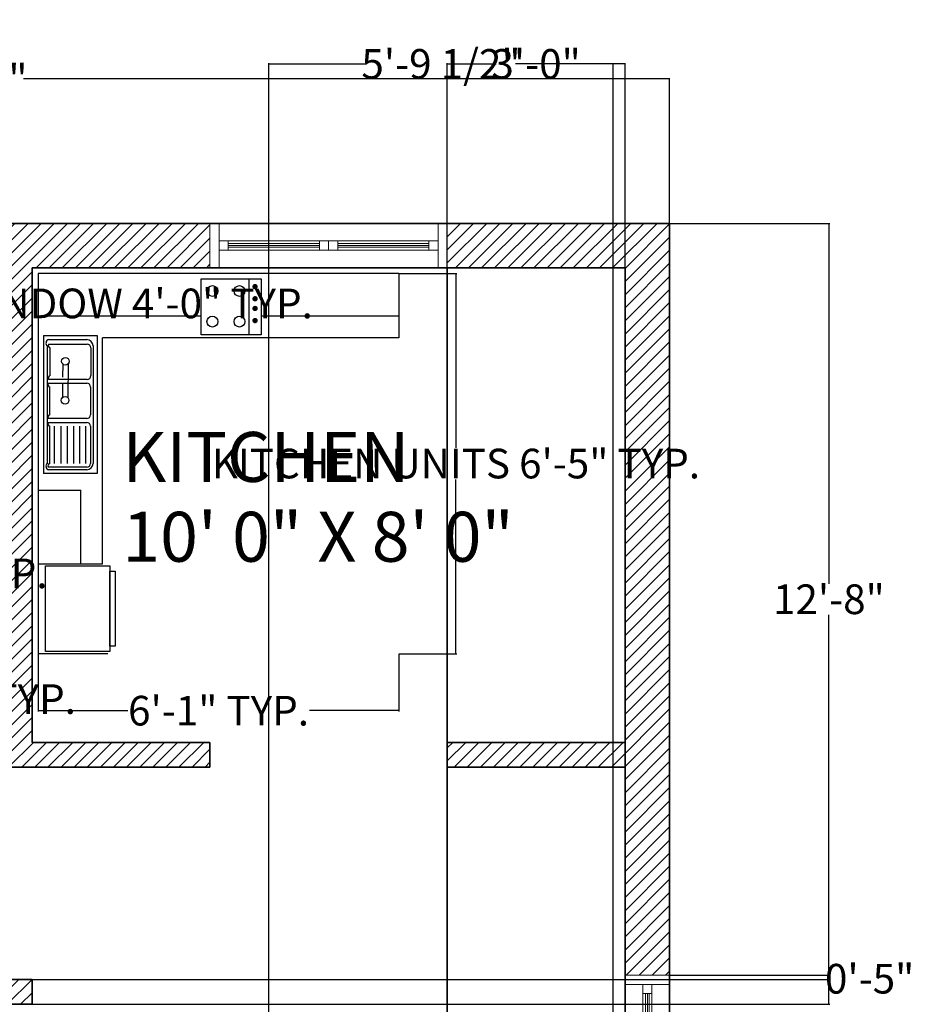
# Model space of a CAD drawing. Units: inches. Extents: x 585 to 1401, y -184 to 463.
# Tile 6 of 8: x 810 to 991, y 264 to 463. Entities that reach past the tile are written whole.
import ezdxf

# ---------------------------------------------------------------- set-up
doc = ezdxf.new("R2010")
doc.units = ezdxf.units.IN
doc.header["$MEASUREMENT"] = 0
for name, color, linetype, lineweight in [('A-ANNO-DIMS', 2, 'Continuous', 18), ('A-AREA-IDEN', 7, 'Continuous', 18), ('A-FLOR-FIXT', 9, 'Continuous', 18), ('A-Glaz', 140, 'Continuous', 18), ('A-Wall', 7, 'Continuous', 35), ('A-WALL-PATT', 252, 'Continuous', 13)]:
    doc.layers.add(name, color=color, linetype=linetype, lineweight=lineweight)
doc.layers.add('TEFRIŞ', color=11, linetype='Continuous')
doc.styles.get("Standard").update_dxf_attribs({"font": 'arial.ttf'})
doc.dimstyles.get("Standard").update_dxf_attribs({"dimtxt": 6, "dimasz": 0.18, "dimexe": 0.18, "dimexo": 0.0625, "dimgap": 0.09, "dimtad": 0, "dimtih": 1, "dimtoh": 1, "dimdec": 0, "dimzin": 0, "dimdsep": 46, "dimlunit": 3, "dimtxsty": 'Standard', "dimblk": 'ARCHTICK', "dimcen": 0.09, "dimadec": 0, "dimazin": 0, "dimtfac": 1, "dimtdec": 0, "dimtofl": 0, "dimtmove": 0, "dimatfit": 3, "dimfxl": 1, "dimtolj": 1, "dimtzin": 0, "dimarcsym": 0})

# ---------------------------------------------------------------- blocks, each defined once
blk = doc.blocks.new('A$C008029BD')
at = {"layer": 'TEFRIŞ', "ltscale": 0.05}
for p, q in [((0, 0), (0, -3.55)), ((3.3699, 0), (0, 0)), ((3.3699, 0), (3.3699, -0.6)), ((1.5225, -0.4), (0, -0.4)), ((3.3699, -0.4), (2.0825, -0.4)), ((0.05, -0.5806), (0.05, -1.8694)), ((0.05, -0.5806), (0.55, -0.5806)), ((0.096, -0.6166), (0.454, -0.6166)), ((0.55, -0.5806), (0.55, -1.8694)), ((0.6, -2.71), (0.6, -0.6)), ((3.3699, -0.6), (0.6, -0.6)), ((0.086, -1.7734), (0.086, -0.6766)), ((0.0991, -0.6595), (0.4571, -0.6595)), ((0.1131, -0.954), (0.1131, -0.6955)), ((0.4931, -0.6955), (0.4931, -0.954)), ((0.514, -0.6766), (0.514, -1.7734)), ((0.2301, -0.8457), (0.2288, -0.9671)), ((0.2801, -0.8455), (0.2768, -1.1584)), ((0.4571, -0.99), (0.0991, -0.99)), ((0.096, -1.0242), (0.454, -1.0242)), ((0.11, -1.3187), (0.11, -1.0602)), ((0.2282, -1.0198), (0.2268, -1.1586)), ((0.49, -1.0602), (0.49, -1.3187)), ((0.454, -1.3547), (0.096, -1.3547)), ((0.096, -1.3912), (0.454, -1.3912)), ((0.11, -1.7734), (0.11, -1.4272)), ((0.1544, -1.7734), (0.1544, -1.4272)), ((0.2144, -1.7734), (0.2144, -1.4272)), ((0.2744, -1.7734), (0.2744, -1.4272)), ((0.3344, -1.7734), (0.3344, -1.4272)), ((0.3902, -1.7734), (0.3902, -1.4272)), ((0.4444, -1.7734), (0.4444, -1.4272)), ((0.49, -1.4272), (0.49, -1.7734)), ((0.454, -1.8094), (0.096, -1.8094)), ((0.454, -1.8334), (0.096, -1.8334)), ((0.55, -1.8694), (0.05, -1.8694)), ((0, -2.025), (0.4, -2.025)), ((0.4, -2.71), (0.4, -2.025)), ((0, -2.71), (0.6, -2.71)), ((0, -3.55), (0.65, -3.55))]:
    blk.add_line(p, q, dxfattribs=at)
at = {"layer": 'TEFRIŞ'}
blk.add_line((1.9688, -0.05), (1.9688, -0.5719), dxfattribs=at)
at = {"layer": 'TEFRIŞ', "ltscale": 0.05}
for points in [[(1.5225, -0.05), (2.0825, -0.05), (2.0825, -0.5719), (1.5225, -0.5719)], [(0.67, -2.73), (0.67, -3.53), (0.07, -3.53), (0.07, -2.73)], [(0.72, -2.78), (0.72, -3.48), (0.67, -3.48), (0.67, -2.78)]]:
    blk.add_lwpolyline(points, close=True, dxfattribs=at)
at = {"layer": 'TEFRIŞ', "const_width": 0.025}
for points in [[(2.0136, -0.1231, 1), (2.0386, -0.1231, 1)], [(2.0136, -0.2361, 1), (2.0386, -0.2361, 1)], [(2.0136, -0.3269, 1), (2.0386, -0.3269, 1)], [(2.0136, -0.4399, 1), (2.0386, -0.4399, 1)]]:
    blk.add_lwpolyline(points, format="xyb", close=True, dxfattribs=at)
at = {"layer": 'TEFRIŞ', "ltscale": 0.05}
for centre, radius in [((1.6277, -0.1636), 0.0505), ((1.6277, -0.4499), 0.0505), ((0.255, -0.8197), 0.036), ((0.2519, -1.1844), 0.036)]:
    blk.add_circle(centre, radius, dxfattribs=at)
at = {"layer": 'TEFRIŞ'}
for centre in [(1.8804, -0.1636), (1.8804, -0.4499)]:
    blk.add_circle(centre, 0.0505, dxfattribs=at)
at = {"layer": 'TEFRIŞ', "ltscale": 0.05}
for centre, radius, start, end in [((0.1083, -0.6495), 0.0351, 110.49764, 230.57771), ((0.454, -0.6766), 0.06, 0, 90), ((0.1177, -0.673), 0.023, 143.98534, 258.51568), ((0.4571, -0.6955), 0.036, 0, 90), ((0.1177, -0.9765), 0.023, 101.48432, 216.01466), ((0.4571, -0.954), 0.036, 270, 0), ((0.1146, -1.0377), 0.023, 143.98534, 258.51568), ((0.454, -1.0602), 0.036, 0, 90), ((0.1146, -1.3412), 0.023, 101.48432, 216.01466), ((0.454, -1.3187), 0.036, 270, 0), ((0.1146, -1.4047), 0.023, 143.98534, 258.51568), ((0.454, -1.4272), 0.036, 0, 90), ((0.1083, -1.8005), 0.0351, 129.42229, 249.50236), ((0.1146, -1.7959), 0.023, 101.48432, 216.01466), ((0.454, -1.7734), 0.06, 270, 0), ((0.454, -1.7734), 0.036, 270, 0)]:
    blk.add_arc(centre, radius, start, end, dxfattribs=at)
blk = doc.blocks.new('_ArchTick')
at = {"color": 0, "linetype": 'ByBlock', "const_width": 0.15}
blk.add_lwpolyline([(-0.5, -0.5), (0.5, 0.5)], dxfattribs=at)
blk = doc.blocks.new('*D28')
at = {"layer": 'A-ANNO-DIMS', "color": 0, "lineweight": -2, "transparency": 16777216}
for p, q in [((654.53, 422.22), (654.53, 451.54)), ((654.53, 451.36), (785.25, 451.36)), ((941.53, 451.36), (810.81, 451.36)), ((941.53, 422.22), (941.53, 451.54))]:
    blk.add_line(p, q, dxfattribs=at)
at = {"layer": 'Defpoints', "color": 0, "transparency": 16777216}
for p in [(941.53, 451.36), (654.53, 422.15), (941.53, 422.15)]:
    blk.add_point(p, dxfattribs=at)
at = {"layer": 'A-ANNO-DIMS', "color": 0, "lineweight": -2, "transparency": 16777216, "xscale": 0.18, "yscale": 0.18, "zscale": 0.18, "rotation": 180}
blk.add_blockref('_ArchTick', (654.53, 451.36), dxfattribs=at)
at = {"layer": 'A-ANNO-DIMS', "color": 0, "lineweight": -2, "transparency": 16777216, "xscale": 0.18, "yscale": 0.18, "zscale": 0.18}
blk.add_blockref('_ArchTick', (941.53, 451.36), dxfattribs=at)
at = {"layer": 'A-ANNO-DIMS', "color": 0, "transparency": 16777216, "insert": (798.03, 451.36), "char_height": 6, "attachment_point": 5}
blk.add_mtext('\\A1;23\'-11"', dxfattribs=at)
blk = doc.blocks.new('WIN-48-DOUBLE-PANEL')
for p, q in [((48, 9), (0, 9)), ((0, 9), (0, 0)), ((1.85, 9), (0, 9)), ((0, 9), (0, 0)), ((1.85, 0), (1.85, 9)), ((1.85, 0), (1.85, 9)), ((46.15, 9), (48, 9)), ((46.15, 0), (46.15, 9)), ((46.15, 0), (46.15, 9)), ((46.15, 0), (46.15, 9)), ((48, 9), (48, 0)), ((48, 0), (48, 9)), ((1.85, 5.44), (46.15, 5.44)), ((3.69, 3.6), (3.69, 5.44)), ((3.69, 4.89), (22.15, 4.89)), ((3.69, 4.52), (22.15, 4.52)), ((3.69, 4.15), (22.15, 4.15)), ((22.15, 5.44), (22.15, 3.6)), ((24, 5.44), (24, 3.6)), ((25.85, 5.44), (25.85, 3.6)), ((44.31, 4.89), (25.85, 4.89)), ((44.31, 4.52), (25.85, 4.52)), ((44.31, 4.15), (25.85, 4.15)), ((44.31, 3.6), (44.31, 5.44)), ((1.85, 3.6), (46.15, 3.6)), ((0, 0), (1.85, 0)), ((48, 0), (0, 0)), ((48, 0), (46.15, 0))]:
    blk.add_line(p, q)
blk = doc.blocks.new('*D38')
at = {"layer": 'A-ANNO-DIMS', "color": 0, "lineweight": -2, "transparency": 16777216}
for p, q in [((711.53, 413.09), (711.53, 405.77)), ((759.53, 413.09), (759.53, 405.77)), ((711.53, 405.95), (759.53, 405.95)), ((759.53, 405.95), (759.71, 405.95))]:
    blk.add_line(p, q, dxfattribs=at)
at = {"layer": 'Defpoints', "color": 0, "transparency": 16777216}
for p in [(711.53, 413.15), (759.53, 413.15), (759.53, 405.95)]:
    blk.add_point(p, dxfattribs=at)
at = {"layer": 'A-ANNO-DIMS', "color": 0, "lineweight": -2, "transparency": 16777216, "xscale": 0.18, "yscale": 0.18, "zscale": 0.18, "rotation": 180}
blk.add_blockref('_ArchTick', (711.53, 405.95), dxfattribs=at)
at = {"layer": 'A-ANNO-DIMS', "color": 0, "lineweight": -2, "transparency": 16777216, "xscale": 0.18, "yscale": 0.18, "zscale": 0.18}
blk.add_blockref('_ArchTick', (759.53, 405.95), dxfattribs=at)
at = {"layer": 'A-ANNO-DIMS', "color": 0, "transparency": 16777216, "insert": (815.89, 405.95), "char_height": 6, "attachment_point": 5}
blk.add_mtext('\\A1;DOUBLE WINDOW 4\'-0" TYP.', dxfattribs=at)
blk = doc.blocks.new('*D50')
at = {"layer": 'A-ANNO-DIMS', "color": 0, "lineweight": -2, "transparency": 16777216}
for p, q in [((770.82, 370.91), (776.81, 370.91)), ((776.63, 370.91), (776.63, 354.54)), ((776.63, 331.78), (776.63, 348.14)), ((770.82, 331.78), (776.81, 331.78))]:
    blk.add_line(p, q, dxfattribs=at)
at = {"layer": 'Defpoints', "color": 0, "transparency": 16777216}
for p in [(770.76, 370.91), (776.63, 370.91), (770.76, 331.78)]:
    blk.add_point(p, dxfattribs=at)
at = {"layer": 'A-ANNO-DIMS', "color": 0, "lineweight": -2, "transparency": 16777216, "xscale": 0.18, "yscale": 0.18, "zscale": 0.18}
for p, rotation in [((776.63, 370.91), 90), ((776.63, 331.78), 270)]:
    blk.add_blockref('_ArchTick', p, dxfattribs=dict(at, rotation=rotation))
at = {"layer": 'A-ANNO-DIMS', "color": 0, "transparency": 16777216, "insert": (776.63, 351.34), "char_height": 6, "attachment_point": 5}
blk.add_mtext('\\A1;LOVESEAT 3\'-3" TYP.', dxfattribs=at)
blk = doc.blocks.new('*D51')
at = {"layer": 'A-ANNO-DIMS', "color": 0, "lineweight": -2, "transparency": 16777216}
for p, q in [((751.2, 331.71), (751.2, 325.73)), ((770.76, 331.71), (770.76, 325.73)), ((751.2, 325.91), (770.76, 325.91)), ((770.76, 325.91), (770.94, 325.91))]:
    blk.add_line(p, q, dxfattribs=at)
at = {"layer": 'Defpoints', "color": 0, "transparency": 16777216}
for p in [(751.2, 331.78), (770.76, 331.78), (770.76, 325.91)]:
    blk.add_point(p, dxfattribs=at)
at = {"layer": 'A-ANNO-DIMS', "color": 0, "lineweight": -2, "transparency": 16777216, "xscale": 0.18, "yscale": 0.18, "zscale": 0.18, "rotation": 180}
blk.add_blockref('_ArchTick', (751.2, 325.91), dxfattribs=at)
at = {"layer": 'A-ANNO-DIMS', "color": 0, "lineweight": -2, "transparency": 16777216, "xscale": 0.18, "yscale": 0.18, "zscale": 0.18}
blk.add_blockref('_ArchTick', (770.76, 325.91), dxfattribs=at)
at = {"layer": 'A-ANNO-DIMS', "color": 0, "transparency": 16777216, "insert": (796.03, 325.91), "char_height": 6, "attachment_point": 5}
blk.add_mtext('\\A1;1\'-7 1/2" TYP.', dxfattribs=at)
blk = doc.blocks.new('*D66')
at = {"layer": 'A-ANNO-DIMS', "color": 0, "lineweight": -2, "transparency": 16777216}
for p, q in [((886.84, 412.01), (898.49, 412.01)), ((898.31, 412.01), (898.31, 376.74)), ((898.31, 335.09), (898.31, 370.36)), ((886.84, 335.09), (898.49, 335.09))]:
    blk.add_line(p, q, dxfattribs=at)
at = {"layer": 'Defpoints', "color": 0, "transparency": 16777216}
for p in [(886.78, 412.01), (898.31, 412.01), (886.78, 335.09)]:
    blk.add_point(p, dxfattribs=at)
at = {"layer": 'A-ANNO-DIMS', "color": 0, "lineweight": -2, "transparency": 16777216, "xscale": 0.18, "yscale": 0.18, "zscale": 0.18}
for p, rotation in [((898.31, 412.01), 90), ((898.31, 335.09), 270)]:
    blk.add_blockref('_ArchTick', p, dxfattribs=dict(at, rotation=rotation))
at = {"layer": 'A-ANNO-DIMS', "color": 0, "transparency": 16777216, "insert": (898.31, 373.55), "char_height": 6, "attachment_point": 5}
blk.add_mtext('\\A1;KITCHEN UNITS 6\'-5" TYP.', dxfattribs=at)
blk = doc.blocks.new('*D67')
at = {"layer": 'A-ANNO-DIMS', "color": 0, "lineweight": -2, "transparency": 16777216}
for p, q in [((813.76, 335.03), (813.76, 323.38)), ((886.78, 335.03), (886.78, 323.38)), ((813.76, 323.56), (831.88, 323.56)), ((886.78, 323.56), (868.66, 323.56))]:
    blk.add_line(p, q, dxfattribs=at)
at = {"layer": 'Defpoints', "color": 0, "transparency": 16777216}
for p in [(813.76, 335.09), (886.78, 335.09), (886.78, 323.56)]:
    blk.add_point(p, dxfattribs=at)
at = {"layer": 'A-ANNO-DIMS', "color": 0, "lineweight": -2, "transparency": 16777216, "xscale": 0.18, "yscale": 0.18, "zscale": 0.18, "rotation": 180}
blk.add_blockref('_ArchTick', (813.76, 323.56), dxfattribs=at)
at = {"layer": 'A-ANNO-DIMS', "color": 0, "lineweight": -2, "transparency": 16777216, "xscale": 0.18, "yscale": 0.18, "zscale": 0.18}
blk.add_blockref('_ArchTick', (886.78, 323.56), dxfattribs=at)
at = {"layer": 'A-ANNO-DIMS', "color": 0, "transparency": 16777216, "insert": (850.27, 323.56), "char_height": 6, "attachment_point": 5}
blk.add_mtext('\\A1;6\'-1" TYP.', dxfattribs=at)
blk = doc.blocks.new('*D78')
at = {"layer": 'A-ANNO-DIMS', "color": 0, "lineweight": -2, "transparency": 16777216}
for p, q in [((860.46, 174.47), (860.46, 454.58)), ((860.46, 454.4), (880.22, 454.4)), ((930.1, 454.4), (910.34, 454.4)), ((930.1, 174.47), (930.1, 454.58))]:
    blk.add_line(p, q, dxfattribs=at)
at = {"layer": 'Defpoints', "color": 0, "transparency": 16777216}
for p in [(930.1, 454.4), (860.46, 174.41), (930.1, 174.41)]:
    blk.add_point(p, dxfattribs=at)
at = {"layer": 'A-ANNO-DIMS', "color": 0, "lineweight": -2, "transparency": 16777216, "xscale": 0.18, "yscale": 0.18, "zscale": 0.18, "rotation": 180}
blk.add_blockref('_ArchTick', (860.46, 454.4), dxfattribs=at)
at = {"layer": 'A-ANNO-DIMS', "color": 0, "lineweight": -2, "transparency": 16777216, "xscale": 0.18, "yscale": 0.18, "zscale": 0.18}
blk.add_blockref('_ArchTick', (930.1, 454.4), dxfattribs=at)
at = {"layer": 'A-ANNO-DIMS', "color": 0, "transparency": 16777216, "insert": (895.28, 454.4), "char_height": 6, "attachment_point": 5}
blk.add_mtext('\\A1;5\'-9 1/2"', dxfattribs=at)
blk = doc.blocks.new('*D83')
at = {"layer": 'A-ANNO-DIMS', "color": 0, "lineweight": -2, "transparency": 16777216}
for p, q in [((896.53, 413.09), (896.53, -175.66)), ((932.53, 413.09), (932.53, -175.66)), ((896.53, -175.48), (906.47, -175.48)), ((932.53, -175.48), (922.59, -175.48))]:
    blk.add_line(p, q, dxfattribs=at)
at = {"layer": 'Defpoints', "color": 0, "transparency": 16777216}
for p in [(896.53, 413.15), (932.53, 413.15), (932.53, -175.48)]:
    blk.add_point(p, dxfattribs=at)
at = {"layer": 'A-ANNO-DIMS', "color": 0, "lineweight": -2, "transparency": 16777216, "xscale": 0.18, "yscale": 0.18, "zscale": 0.18, "rotation": 180}
blk.add_blockref('_ArchTick', (896.53, -175.48), dxfattribs=at)
at = {"layer": 'A-ANNO-DIMS', "color": 0, "lineweight": -2, "transparency": 16777216, "xscale": 0.18, "yscale": 0.18, "zscale": 0.18}
blk.add_blockref('_ArchTick', (932.53, -175.48), dxfattribs=at)
at = {"layer": 'A-ANNO-DIMS', "color": 0, "transparency": 16777216, "insert": (914.53, -175.48), "char_height": 6, "attachment_point": 5}
blk.add_mtext('\\A1;3\'-0"', dxfattribs=at)
blk = doc.blocks.new('*D84')
at = {"layer": 'A-ANNO-DIMS', "color": 0, "lineweight": -2, "transparency": 16777216}
for p, q in [((941.59, 422.15), (973.96, 422.15)), ((973.78, 422.15), (973.78, 349.25)), ((973.78, 270.04), (973.78, 342.95)), ((941.59, 270.04), (973.96, 270.04))]:
    blk.add_line(p, q, dxfattribs=at)
at = {"layer": 'Defpoints', "color": 0, "transparency": 16777216}
for p in [(941.53, 422.15), (973.78, 422.15), (941.53, 270.04)]:
    blk.add_point(p, dxfattribs=at)
at = {"layer": 'A-ANNO-DIMS', "color": 0, "lineweight": -2, "transparency": 16777216, "xscale": 0.18, "yscale": 0.18, "zscale": 0.18}
for p, rotation in [((973.78, 422.15), 90), ((973.78, 270.04), 270)]:
    blk.add_blockref('_ArchTick', p, dxfattribs=dict(at, rotation=rotation))
at = {"layer": 'A-ANNO-DIMS', "color": 0, "transparency": 16777216, "insert": (973.78, 346.1), "char_height": 6, "attachment_point": 5}
blk.add_mtext('\\A1;12\'-8"', dxfattribs=at)
blk = doc.blocks.new('*D88')
at = {"layer": 'A-ANNO-DIMS', "color": 0, "lineweight": -2, "transparency": 16777216}
for p, q in [((896.53, -134.17), (896.53, 454.58)), ((896.53, 454.4), (906.47, 454.4)), ((932.53, 454.4), (922.59, 454.4)), ((932.53, -134.17), (932.53, 454.58))]:
    blk.add_line(p, q, dxfattribs=at)
at = {"layer": 'Defpoints', "color": 0, "transparency": 16777216}
for p in [(932.53, 454.4), (896.53, -134.23), (932.53, -134.23)]:
    blk.add_point(p, dxfattribs=at)
at = {"layer": 'A-ANNO-DIMS', "color": 0, "lineweight": -2, "transparency": 16777216, "xscale": 0.18, "yscale": 0.18, "zscale": 0.18, "rotation": 180}
blk.add_blockref('_ArchTick', (896.53, 454.4), dxfattribs=at)
at = {"layer": 'A-ANNO-DIMS', "color": 0, "lineweight": -2, "transparency": 16777216, "xscale": 0.18, "yscale": 0.18, "zscale": 0.18}
blk.add_blockref('_ArchTick', (932.53, 454.4), dxfattribs=at)
at = {"layer": 'A-ANNO-DIMS', "color": 0, "transparency": 16777216, "insert": (914.53, 454.4), "char_height": 6, "attachment_point": 5}
blk.add_mtext('\\A1;3\'-0"', dxfattribs=at)
blk = doc.blocks.new('*D89')
at = {"layer": 'A-ANNO-DIMS', "color": 0, "lineweight": -2, "transparency": 16777216}
for p, q in [((812.59, 269.15), (973.96, 269.15)), ((973.78, 269.15), (973.78, 269.33)), ((973.78, 269.33), (973.96, 269.33)), ((973.78, 264.15), (973.78, 269.15)), ((812.59, 264.15), (973.96, 264.15))]:
    blk.add_line(p, q, dxfattribs=at)
at = {"layer": 'Defpoints', "color": 0, "transparency": 16777216}
for p in [(812.53, 269.15), (973.78, 269.15), (812.53, 264.15)]:
    blk.add_point(p, dxfattribs=at)
at = {"layer": 'A-ANNO-DIMS', "color": 0, "lineweight": -2, "transparency": 16777216, "xscale": 0.18, "yscale": 0.18, "zscale": 0.18}
for p, rotation in [((973.78, 269.15), 90), ((973.78, 264.15), 270)]:
    blk.add_blockref('_ArchTick', p, dxfattribs=dict(at, rotation=rotation))
at = {"layer": 'A-ANNO-DIMS', "color": 0, "transparency": 16777216, "insert": (982.02, 269.33), "char_height": 6, "attachment_point": 5}
blk.add_mtext('\\A1;0\'-5"', dxfattribs=at)

msp = doc.modelspace()

# ---------------------------------------------------------------- hatches: boundary and pattern name
at = {"layer": 'A-WALL-PATT'}
h = msp.add_hatch(dxfattribs=at)
h.set_pattern_fill('ANSI31', color=256, scale=15)
h.set_pattern_definition([(45, (599.059, -1e-14), (-1.325825, 1.325825), [])])
h.paths.add_polyline_path([(711.53, 422.15), (654.53, 422.15), (654.53, -109.85), (680.03, -109.85), (680.03, -100.85), (663.53, -100.85), (663.53, 48.87), (759.53, 48.87), (759.53, 57.87), (663.53, 57.87), (663.53, 144.15), (663.53, 264.15), (812.53, 264.15), (812.53, 269.15), (663.53, 269.15), (663.53, 413.15), (711.53, 413.15)])
h.paths.add_polyline_path([(753.53, -100.85), (728.03, -100.85), (728.03, -109.85), (753.53, -109.85)], flags=17)
h.paths.add_polyline_path([(812.53, -71.54), (807.53, -71.54), (807.53, -100.85), (795.53, -100.85), (795.53, -109.85), (807.53, -109.85), (807.53, -143.23), (848.53, -143.23), (848.53, -134.23), (812.53, -134.23)])
h.paths.add_polyline_path([(941.53, 8.77), (932.53, 8.77), (932.53, -9.23), (812.53, -9.23), (812.53, 5.77), (807.53, 5.77), (807.53, -29.54), (812.53, -29.54), (812.53, -14.23), (932.53, -14.23), (932.53, -134.23), (896.53, -134.23), (896.53, -143.23), (941.53, -143.23)])
h.paths.add_polyline_path([(941.53, 91.77), (932.53, 91.77), (932.53, 55.77), (812.53, 55.77), (812.53, 98.58), (807.53, 98.58), (807.53, 35.77), (812.53, 35.77), (812.53, 50.77), (932.53, 50.77), (932.53, 32.77), (941.53, 32.77)])
h.paths.add_polyline_path([(941.53, 222.04), (932.53, 222.04), (932.53, 180.77), (807.53, 180.77), (807.53, 140.58), (812.53, 140.58), (812.53, 175.77), (932.53, 175.77), (932.53, 139.77), (941.53, 139.77)])
h.paths.add_polyline_path([(941.53, 422.15), (896.53, 422.15), (896.53, 413.15), (932.53, 413.15), (932.53, 317.15), (896.53, 317.15), (896.53, 312.15), (932.53, 312.15), (932.53, 270.04), (941.53, 270.04)])
h.paths.add_polyline_path([(848.53, 422.15), (759.53, 422.15), (759.53, 413.15), (807.53, 413.15), (807.53, 312.15), (848.53, 312.15), (848.53, 317.15), (812.53, 317.15), (812.53, 413.15), (848.53, 413.15)])

# ---------------------------------------------------------------- linework, layer by layer
at = {"layer": 'A-Wall'}
for p, q in [((654.53, 422.15), (941.53, 422.15)), ((941.53, 422.15), (941.53, -143.23)), ((812.53, 413.15), (812.53, 317.15)), ((812.53, 413.15), (932.53, 413.15)), ((932.53, 413.15), (932.53, 317.15)), ((812.53, 317.15), (848.53, 317.15)), ((848.53, 317.15), (848.53, 312.15)), ((896.53, 317.15), (896.53, 312.15)), ((896.53, 317.15), (932.53, 317.15)), ((807.53, 312.15), (848.53, 312.15)), ((896.53, 312.15), (932.53, 312.15)), ((932.53, 312.15), (932.53, 180.77)), ((663.53, 269.15), (812.53, 269.15)), ((812.53, 269.15), (812.53, 264.15)), ((663.53, 264.15), (812.53, 264.15))]:
    msp.add_line(p, q, dxfattribs=at)

# ---------------------------------------------------------------- block references
at = {"layer": 'A-FLOR-FIXT', "xscale": 21.66627528827239, "yscale": 21.66627528827239, "zscale": 21.66627528827239}
msp.add_blockref('A$C008029BD', (813.76, 412.01), dxfattribs=at)
at = {"layer": 'A-Glaz'}
msp.add_blockref('WIN-48-DOUBLE-PANEL', (848.53, 413.15), dxfattribs=at)
at = {"layer": 'A-Glaz', "rotation": 270.0000000000021}
msp.add_blockref('WIN-48-DOUBLE-PANEL', (932.53, 270.04), dxfattribs=at)

# ---------------------------------------------------------------- texts
at = {"layer": 'A-AREA-IDEN'}
for s, height, p in [('KITCHEN', 10.101, (830.8, 369.84)), ('10\' 0" X 8\' 0"', 10.1013, (830.8, 353.69))]:
    msp.add_text(s, height=height, dxfattribs=at).set_placement(p)

# ---------------------------------------------------------------- dimensions: what is measured, and where the dimension line sits
at = {"layer": 'A-ANNO-DIMS'}
for base, p1, p2, override, picture, middle in [((930.1, 454.4), (860.46, 174.41), (930.1, 174.41), {"dimdec": 1, "dimlfac": 1, "dimrnd": 0, "dimzin": 1, "dimdsep": 46, "dimlunit": 4, "dimfrac": 2}, '*D78', (895.28, 454.4)), ((932.53, 454.4), (896.53, -134.23), (932.53, -134.23), {"dimdec": 1, "dimlfac": 1, "dimrnd": 0, "dimzin": 1, "dimdsep": 46, "dimlunit": 4, "dimfrac": 2}, '*D88', (914.53, 454.4)), ((941.53, 451.36), (654.53, 422.15), (941.53, 422.15), {"dimclrd": 0, "dimclre": 0, "dimclrt": 0}, '*D28', (798.03, 451.36)), ((932.53, -175.48), (896.53, 413.15), (932.53, 413.15), {"dimdec": 1, "dimlfac": 1, "dimrnd": 0, "dimzin": 1, "dimdsep": 46, "dimlunit": 4, "dimfrac": 2}, '*D83', (914.53, -175.48))]:
    dim = msp.add_linear_dim(base=base, p1=p1, p2=p2, dimstyle='Standard', override=override, dxfattribs=at)
    dim.commit()
    dim.dimension.update_dxf_attribs({"geometry": picture, "text_midpoint": middle})
for base, p1, p2, text, picture, middle in [((759.53, 405.95), (711.53, 413.15), (759.53, 413.15), 'DOUBLE WINDOW <> TYP.', '*D38', (815.89, 405.95)), ((886.78, 323.56), (813.76, 335.09), (886.78, 335.09), '<> TYP.', '*D67', (850.27, 323.56))]:
    dim = msp.add_linear_dim(base=base, p1=p1, p2=p2, text=text, dimstyle='Standard', override={"dimdec": 1, "dimlfac": 1, "dimrnd": 0, "dimzin": 1, "dimdsep": 46, "dimlunit": 4, "dimfrac": 2}, dxfattribs=at)
    dim.commit()
    dim.dimension.update_dxf_attribs({"geometry": picture, "text_midpoint": middle})
for base, p1, p2, picture, middle in [((973.78, 422.15), (941.53, 270.04), (941.53, 422.15), '*D84', (973.78, 346.1)), ((973.78, 269.15), (812.53, 264.15), (812.53, 269.15), '*D89', (982.02, 269.33))]:
    dim = msp.add_linear_dim(base=base, p1=p1, p2=p2, angle=90, dimstyle='Standard', override={"dimdec": 1, "dimlfac": 1, "dimrnd": 0, "dimzin": 1, "dimdsep": 46, "dimlunit": 4, "dimfrac": 2}, dxfattribs=at)
    dim.commit()
    dim.dimension.update_dxf_attribs({"geometry": picture, "text_midpoint": middle})
for base, p1, p2, angle, text, picture, middle in [((898.31, 412.01), (886.78, 335.09), (886.78, 412.01), 90, 'KITCHEN UNITS <> TYP.', '*D66', (898.31, 373.55)), ((776.63, 370.91), (770.76, 331.78), (770.76, 370.91), 90, 'LOVESEAT <> TYP.', '*D50', (776.63, 351.34)), ((770.76, 325.91), (751.2, 331.78), (770.76, 331.78), 0, '<> TYP.', '*D51', (796.03, 325.91))]:
    dim = msp.add_linear_dim(base=base, p1=p1, p2=p2, angle=angle, text=text, dimstyle='Standard', override={"dimdec": 1, "dimlfac": 1, "dimrnd": 0, "dimzin": 1, "dimdsep": 46, "dimlunit": 4, "dimfrac": 2}, dxfattribs=at)
    dim.commit()
    dim.dimension.update_dxf_attribs({"geometry": picture, "text_midpoint": middle})

doc.saveas('drawing.dxf')
